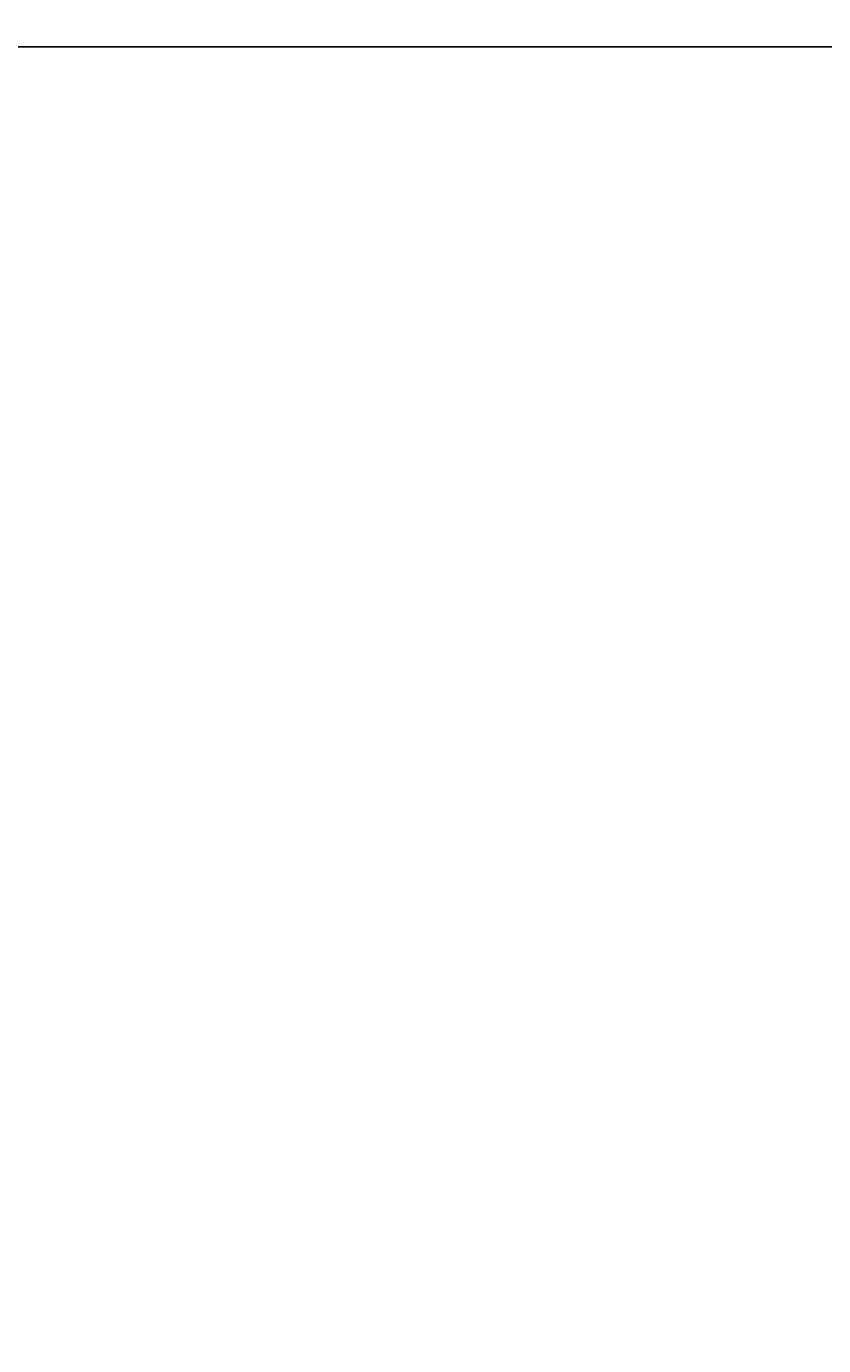
# Model space of a CAD drawing. Units: inches. Extents: x -61 to 1599, y -1316 to 257.
# Tile 24 of 204: x 365 to 388, y -912 to -873. Entities that reach past the tile are written whole.
import ezdxf

# ---------------------------------------------------------------- set-up
doc = ezdxf.new("R2010")
doc.units = ezdxf.units.IN
doc.header["$MEASUREMENT"] = 0
doc.layers.add('A-ANNO-DIMS', color=2, linetype='Continuous', lineweight=18)
doc.styles.get("Standard").update_dxf_attribs({"font": 'arial.ttf'})
doc.dimstyles.get("Standard").update_dxf_attribs({"dimtxt": 0.18, "dimasz": 0.18, "dimexe": 0.18, "dimexo": 0.0625, "dimgap": 0.09, "dimtad": 0, "dimtih": 1, "dimtoh": 1, "dimdec": 0, "dimzin": 0, "dimdsep": 46, "dimlunit": 3, "dimtxsty": 'Standard', "dimcen": 0.09, "dimadec": 0, "dimazin": 0, "dimtfac": 1, "dimtdec": 0, "dimtofl": 0, "dimtmove": 0, "dimatfit": 3, "dimfxl": 1, "dimtolj": 1, "dimtzin": 0, "dimarcsym": 0})

# ---------------------------------------------------------------- blocks, each defined once
blk = doc.blocks.new('*D696')
at = {"layer": 'A-ANNO-DIMS', "color": 0, "lineweight": -2, "transparency": 16777216}
for p, q in [((690.64, -873.169), (-61.077, -873.169)), ((-60.897, -873.349), (-60.897, -1025.799)), ((-60.897, -1178.613), (-60.897, -1026.163)), ((690.64, -1178.793), (-61.077, -1178.793))]:
    blk.add_line(p, q, dxfattribs=at)
at = {"layer": 'A-ANNO-DIMS', "color": 0, "transparency": 16777216}
for points in [[(-60.927, -873.349), (-60.867, -873.349), (-60.897, -873.169)], [(-60.927, -1178.613), (-60.867, -1178.613), (-60.897, -1178.793)]]:
    blk.add_solid(points, dxfattribs=at)
at = {"layer": 'DEFPOINTS', "color": 0, "transparency": 16777216}
for p in [(-60.897, -873.169), (690.703, -873.169), (690.703, -1178.793)]:
    blk.add_point(p, dxfattribs=at)
at = {"layer": 'A-ANNO-DIMS', "color": 0, "transparency": 16777216, "insert": (-60.897, -1025.981), "char_height": 0.18, "attachment_point": 5}
blk.add_mtext('\\A1;305.6', dxfattribs=at)
blk = doc.blocks.new('*D710')
at = {"layer": 'A-ANNO-DIMS', "color": 0, "lineweight": -2, "transparency": 16777216}
for p, q in [((319.703, -465.385), (319.703, -1315.725)), ((403.703, -465.385), (403.703, -1315.725)), ((319.883, -1315.545), (361.484, -1315.545)), ((403.523, -1315.545), (361.921, -1315.545))]:
    blk.add_line(p, q, dxfattribs=at)
at = {"layer": 'A-ANNO-DIMS', "color": 0, "transparency": 16777216}
for points in [[(319.883, -1315.515), (319.883, -1315.575), (319.703, -1315.545)], [(403.523, -1315.515), (403.523, -1315.575), (403.703, -1315.545)]]:
    blk.add_solid(points, dxfattribs=at)
at = {"layer": 'DEFPOINTS', "color": 0, "transparency": 16777216}
for p in [(319.703, -465.323), (403.703, -465.323), (403.703, -1315.545)]:
    blk.add_point(p, dxfattribs=at)
at = {"layer": 'A-ANNO-DIMS', "color": 0, "transparency": 16777216, "insert": (361.703, -1315.545), "char_height": 0.18, "attachment_point": 5}
blk.add_mtext('\\A1;84', dxfattribs=at)

msp = doc.modelspace()

# ---------------------------------------------------------------- dimensions: what is measured, and where the dimension line sits
at = {"layer": 'A-ANNO-DIMS'}
dim = msp.add_linear_dim(base=(403.7028, -1315.5446), p1=(319.7028, -465.3229), p2=(403.7028, -465.3229), dimstyle='Standard', override={"dimdec": 0, "dimlfac": 1, "dimrnd": 0, "dimzin": 0, "dimdsep": 46, "dimlunit": 2}, dxfattribs=at)
dim.commit()
dim.dimension.update_dxf_attribs({"geometry": '*D710', "text_midpoint": (361.7028, -1315.5446)})
dim = msp.add_linear_dim(base=(-60.8972, -873.169), p1=(690.7028, -1178.7933), p2=(690.7028, -873.169), angle=90, dimstyle='Standard', override={"dimdec": 1, "dimlfac": 1, "dimrnd": 0, "dimzin": 0, "dimdsep": 46, "dimlunit": 2}, dxfattribs=at)
dim.commit()
dim.dimension.update_dxf_attribs({"geometry": '*D696', "text_midpoint": (-60.8972, -1025.9812)})

doc.saveas('drawing.dxf')
